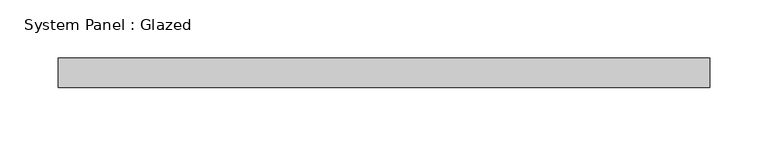
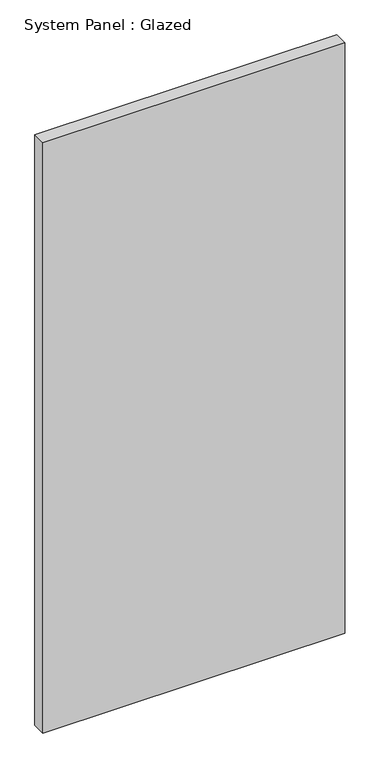
"""IFC4 building model written with IfcOpenShell, lengths in millimetres: plate geometry, System Panel : Glazed."""

from ifc_helpers import new_model, si_unit, origin, origin_with_axes, place, context, project, spatial, polyline, outline, extrude, source, transform, mapped, element, save


def system_panel_glazed_b34e3459(model_context):
    return source(origin(), model_context, "Body", "SweptSolid", [
        extrude(outline(polyline([(279.4, 19.05), (-279.4, 19.05), (-279.4, 44.45), (279.4, 44.45), (279.4, 19.05)])), origin_with_axes(), (0.0, 0.0, 1.0), 1155.7),
    ])


if __name__ == "__main__":
    model = new_model("IFC4")
    model_context = context("Model", 3, world=origin())
    ifc_project = project(units=[si_unit("LENGTHUNIT", "METRE", prefix="MILLI")], contexts=[model_context])
    site = spatial("IfcSite", under=ifc_project)
    building = spatial("IfcBuilding", under=site)
    placement = place(None, origin())
    system_panel_glazed_shape = system_panel_glazed_b34e3459(model_context)
    element("IfcPlate", 1, ObjectType="System Panel : Glazed", at=placement, inside=building, context=model_context, shape_type="MappedRepresentation", body=[
        mapped(system_panel_glazed_shape, transform((0.0, 0.0, 0.0), x_axis=(1.0, 0.0, 0.0), y_axis=(0.0, 1.0, 0.0), z_axis=(0.0, 0.0, 1.0))),
    ])
    save(model, "model.ifc")

# Revit data of these elements
# Type "System Panel : Glazed"
#   Construction Type Id = "GSP4R"
#   Analytic Construction = "1/8 in Pilkington single glazing"
#   Visual Light Transmittance = 0.9
#   Solar Heat Gain Coefficient = 0.86
#   Heat Transfer Coefficient (U) = 1.18115 BTU/(h·ft²·°F)
# Element 1 (IfcPlate, "System Panel : Glazed")
#   Materials on its faces: "Glass"
# Materials
#   "Glass": class "Glass", colour RGB 0 128 192, transparency 0.75, Description = "Soda Lime Glass", Cost = 0
